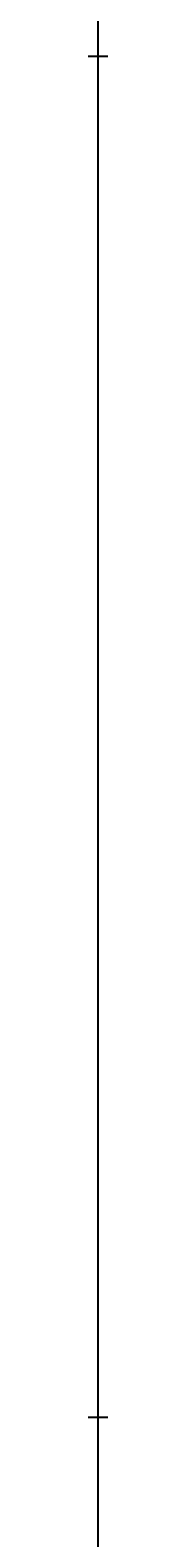
# Model space of a CAD drawing. Units: inches. Extents: x 35362 to 73946, y 43607 to 67532.
# Tile 32 of 134: x 48373 to 48373, y 46091 to 46564. Entities that reach past the tile are written whole.
import ezdxf

# ---------------------------------------------------------------- set-up
doc = ezdxf.new("R2010")
doc.units = ezdxf.units.IN
doc.header["$MEASUREMENT"] = 0
doc.layers.add('A-ANNO-DIMS', color=2, linetype='Continuous', lineweight=18)
doc.styles.get("Standard").update_dxf_attribs({"font": 'arial.ttf'})
doc.dimstyles.get("Standard").update_dxf_attribs({"dimtxt": 0.18, "dimasz": 0.18, "dimexe": 0.18, "dimexo": 0.0625, "dimgap": 0.09, "dimtad": 0, "dimtih": 1, "dimtoh": 1, "dimdec": 4, "dimzin": 0, "dimdsep": 46, "dimtxsty": 'Standard', "dimcen": 0.09, "dimadec": 0, "dimazin": 0, "dimtfac": 1, "dimtdec": 4, "dimtofl": 0, "dimtmove": 0, "dimatfit": 3, "dimfxl": 1, "dimtolj": 1, "dimtzin": 0, "dimarcsym": 0})

# ---------------------------------------------------------------- blocks, each defined once
blk = doc.blocks.new('*D5')
at = {"layer": 'A-ANNO-DIMS', "color": 0, "lineweight": -2, "transparency": 16777216}
for p, q in [((37121.95, 46919.32), (37121.95, 43606.68)), ((69871.5, 45449.83), (69871.5, 43606.68)), ((37122.13, 43606.86), (53496.29, 43606.86)), ((69871.32, 43606.86), (53497.15, 43606.86))]:
    blk.add_line(p, q, dxfattribs=at)
at = {"layer": 'A-ANNO-DIMS', "color": 0, "transparency": 16777216}
for points in [[(37122.13, 43606.89), (37122.13, 43606.83), (37121.95, 43606.86)], [(69871.32, 43606.89), (69871.32, 43606.83), (69871.5, 43606.86)]]:
    blk.add_solid(points, dxfattribs=at)
at = {"layer": 'Defpoints', "color": 0, "transparency": 16777216}
for p in [(37121.95, 46919.38), (69871.5, 45449.89), (69871.5, 43606.86)]:
    blk.add_point(p, dxfattribs=at)
at = {"layer": 'A-ANNO-DIMS', "color": 0, "transparency": 16777216, "insert": (53496.72, 43606.86), "char_height": 0.18, "attachment_point": 5}
blk.add_mtext('\\A1;32750', dxfattribs=at)
blk = doc.blocks.new('*D11')
at = {"layer": 'A-ANNO-DIMS', "color": 0, "lineweight": -2, "transparency": 16777216}
for p, q in [((47978.66, 56028.77), (47978.66, 43606.68)), ((53109.76, 56028.77), (53109.76, 43606.68)), ((47978.84, 43606.86), (50543.87, 43606.86)), ((53109.58, 43606.86), (50544.55, 43606.86))]:
    blk.add_line(p, q, dxfattribs=at)
at = {"layer": 'A-ANNO-DIMS', "color": 0, "transparency": 16777216}
for points in [[(47978.84, 43606.89), (47978.84, 43606.83), (47978.66, 43606.86)], [(53109.58, 43606.89), (53109.58, 43606.83), (53109.76, 43606.86)]]:
    blk.add_solid(points, dxfattribs=at)
at = {"layer": 'Defpoints', "color": 0, "transparency": 16777216}
for p in [(47978.66, 56028.84), (53109.76, 56028.84), (53109.76, 43606.86)]:
    blk.add_point(p, dxfattribs=at)
at = {"layer": 'A-ANNO-DIMS', "color": 0, "transparency": 16777216, "insert": (50544.21, 43606.86), "char_height": 0.18, "attachment_point": 5}
blk.add_mtext('\\A1;5131', dxfattribs=at)
blk = doc.blocks.new('*D27')
at = {"layer": 'A-ANNO-DIMS', "color": 0, "lineweight": -2, "transparency": 16777216}
for p, q in [((47978.66, 56028.77), (47978.66, 43606.68)), ((48373.49, 53428.96), (48373.49, 43606.68)), ((47978.84, 43606.86), (48175.68, 43606.86)), ((48373.31, 43606.86), (48176.47, 43606.86))]:
    blk.add_line(p, q, dxfattribs=at)
at = {"layer": 'A-ANNO-DIMS', "color": 0, "transparency": 16777216}
for points in [[(47978.84, 43606.89), (47978.84, 43606.83), (47978.66, 43606.86)], [(48373.31, 43606.89), (48373.31, 43606.83), (48373.49, 43606.86)]]:
    blk.add_solid(points, dxfattribs=at)
at = {"layer": 'Defpoints', "color": 0, "transparency": 16777216}
for p in [(47978.66, 56028.84), (48373.49, 53429.02), (48373.49, 43606.86)]:
    blk.add_point(p, dxfattribs=at)
at = {"layer": 'A-ANNO-DIMS', "color": 0, "transparency": 16777216, "insert": (48176.08, 43606.86), "char_height": 0.18, "attachment_point": 5}
blk.add_mtext('\\A1;394.8', dxfattribs=at)
blk = doc.blocks.new('*D67')
at = {"layer": 'A-ANNO-DIMS', "color": 0, "lineweight": -2, "transparency": 16777216}
for p, q in [((56873.54, 53351.53), (35361.77, 53351.53)), ((35361.95, 53351.35), (35361.95, 49400.89)), ((35361.95, 45450.07), (35361.95, 49400.53)), ((53793.58, 45449.89), (35361.77, 45449.89))]:
    blk.add_line(p, q, dxfattribs=at)
at = {"layer": 'A-ANNO-DIMS', "color": 0, "transparency": 16777216}
for points in [[(35361.92, 53351.35), (35361.98, 53351.35), (35361.95, 53351.53)], [(35361.92, 45450.07), (35361.98, 45450.07), (35361.95, 45449.89)]]:
    blk.add_solid(points, dxfattribs=at)
at = {"layer": 'Defpoints', "color": 0, "transparency": 16777216}
for p in [(35361.95, 53351.53), (56873.6, 53351.53), (53793.64, 45449.89)]:
    blk.add_point(p, dxfattribs=at)
at = {"layer": 'A-ANNO-DIMS', "color": 0, "transparency": 16777216, "insert": (35361.95, 49400.71), "char_height": 0.18, "attachment_point": 5}
blk.add_mtext('\\A1;7901.6', dxfattribs=at)
blk = doc.blocks.new('*D76')
at = {"layer": 'A-ANNO-DIMS', "color": 0, "lineweight": -2, "transparency": 16777216}
for p, q in [((54052.84, 46555.29), (35361.77, 46555.29)), ((35361.95, 46555.11), (35361.95, 46342.27)), ((35361.95, 46129.06), (35361.95, 46341.9)), ((53793.58, 46128.88), (35361.77, 46128.88))]:
    blk.add_line(p, q, dxfattribs=at)
at = {"layer": 'A-ANNO-DIMS', "color": 0, "transparency": 16777216}
for points in [[(35361.92, 46555.11), (35361.98, 46555.11), (35361.95, 46555.29)], [(35361.92, 46129.06), (35361.98, 46129.06), (35361.95, 46128.88)]]:
    blk.add_solid(points, dxfattribs=at)
at = {"layer": 'Defpoints', "color": 0, "transparency": 16777216}
for p in [(35361.95, 46555.29), (54052.9, 46555.29), (53793.64, 46128.88)]:
    blk.add_point(p, dxfattribs=at)
at = {"layer": 'A-ANNO-DIMS', "color": 0, "transparency": 16777216, "insert": (35361.95, 46342.09), "char_height": 0.18, "attachment_point": 5}
blk.add_mtext('\\A1;426.4', dxfattribs=at)
blk = doc.blocks.new('*D90')
at = {"layer": 'A-ANNO-DIMS', "color": 0, "lineweight": -2, "transparency": 16777216}
for p, q in [((53707.72, 47291.29), (35361.77, 47291.29)), ((35361.95, 47291.11), (35361.95, 46710.26)), ((35361.95, 46129.06), (35361.95, 46709.9)), ((53793.58, 46128.88), (35361.77, 46128.88))]:
    blk.add_line(p, q, dxfattribs=at)
at = {"layer": 'A-ANNO-DIMS', "color": 0, "transparency": 16777216}
for points in [[(35361.92, 47291.11), (35361.98, 47291.11), (35361.95, 47291.29)], [(35361.92, 46129.06), (35361.98, 46129.06), (35361.95, 46128.88)]]:
    blk.add_solid(points, dxfattribs=at)
at = {"layer": 'Defpoints', "color": 0, "transparency": 16777216}
for p in [(53707.78, 47291.29), (35361.95, 46128.88), (53793.64, 46128.88)]:
    blk.add_point(p, dxfattribs=at)
at = {"layer": 'A-ANNO-DIMS', "color": 0, "transparency": 16777216, "insert": (35361.95, 46710.08), "char_height": 0.18, "attachment_point": 5}
blk.add_mtext('\\A1;1162.4', dxfattribs=at)

msp = doc.modelspace()

# ---------------------------------------------------------------- dimensions: what is measured, and where the dimension line sits
at = {"layer": 'A-ANNO-DIMS'}
for base, p1, p2, override, picture, middle in [((53109.76, 43606.859), (47978.665, 56028.836), (53109.76, 56028.836), {"dimdec": 0, "dimlfac": 1, "dimrnd": 0, "dimzin": 0, "dimdsep": 46, "dimlunit": 2}, '*D11', (50544.212, 43606.859)), ((48373.492, 43606.859), (47978.665, 56028.836), (48373.492, 53429.019), {"dimdec": 1, "dimlfac": 1, "dimrnd": 0, "dimzin": 0, "dimdsep": 46, "dimlunit": 2}, '*D27', (48176.078, 43606.859)), ((69871.496, 43606.859), (37121.949, 46919.381), (69871.496, 45449.894), {"dimdec": 0, "dimlfac": 1, "dimrnd": 0, "dimzin": 0, "dimdsep": 46, "dimlunit": 2}, '*D5', (53496.723, 43606.859))]:
    dim = msp.add_linear_dim(base=base, p1=p1, p2=p2, dimstyle='Standard', override=override, dxfattribs=at)
    dim.commit()
    dim.dimension.update_dxf_attribs({"geometry": picture, "text_midpoint": middle})
for base, p1, p2, picture, middle in [((35361.949, 53351.529), (53793.638, 45449.894), (56873.602, 53351.529), '*D67', (35361.949, 49400.712)), ((35361.949, 46128.878), (53707.781, 47291.285), (53793.638, 46128.878), '*D90', (35361.949, 46710.081)), ((35361.949, 46555.293), (53793.638, 46128.878), (54052.899, 46555.293), '*D76', (35361.949, 46342.086))]:
    dim = msp.add_linear_dim(base=base, p1=p1, p2=p2, angle=90, dimstyle='Standard', override={"dimdec": 1, "dimlfac": 1, "dimrnd": 0, "dimzin": 0, "dimdsep": 46, "dimlunit": 2}, dxfattribs=at)
    dim.commit()
    dim.dimension.update_dxf_attribs({"geometry": picture, "text_midpoint": middle})

doc.saveas('drawing.dxf')
